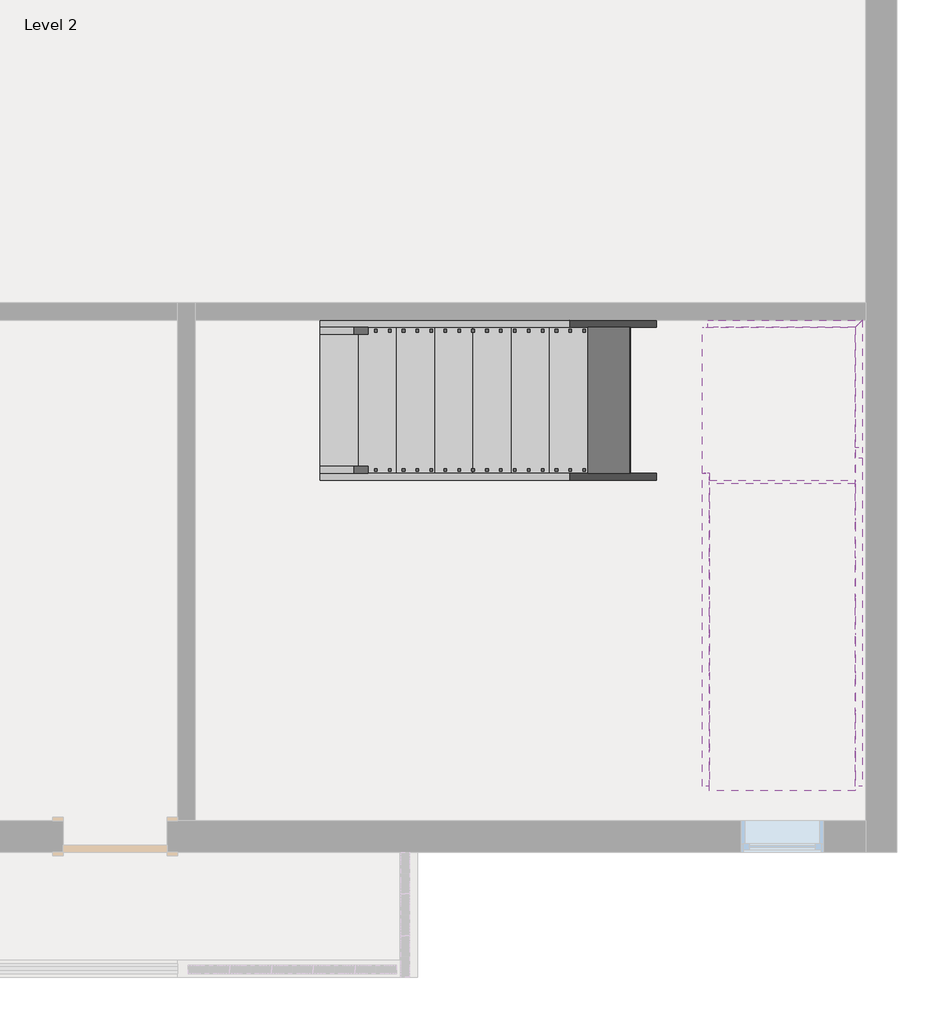
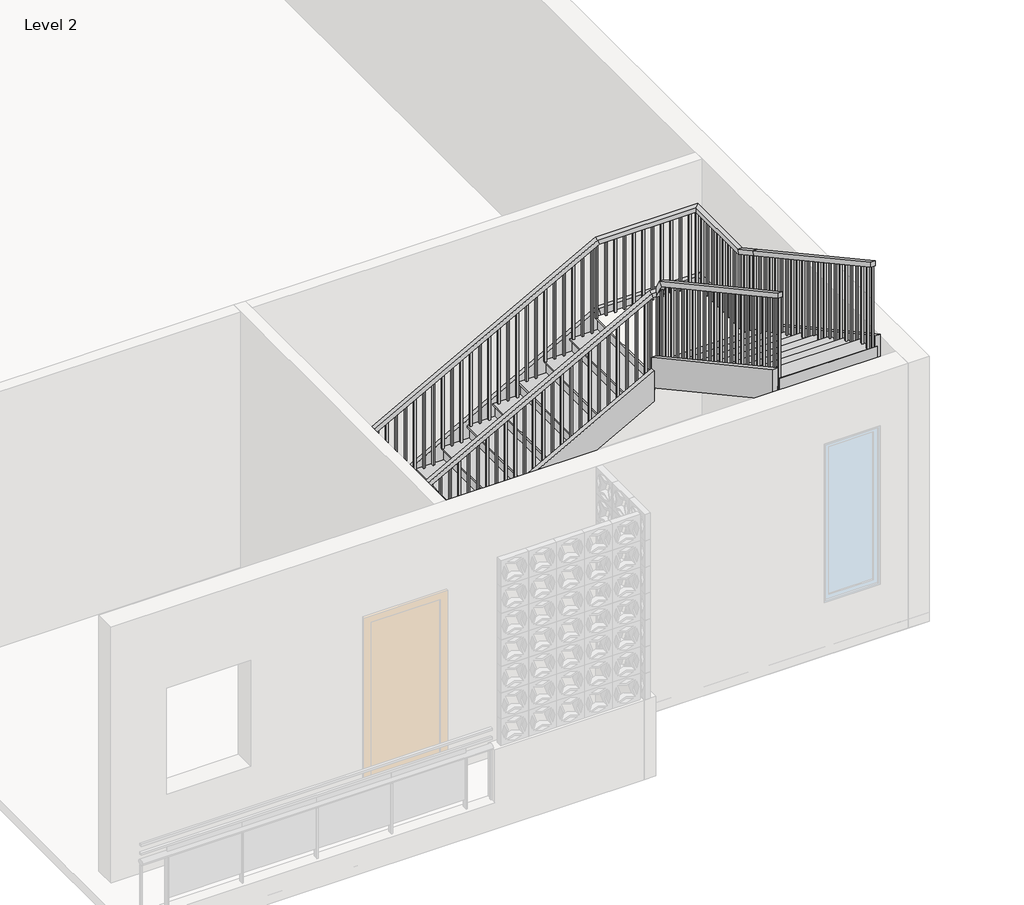
# One storey, part 2 of 2: 6 members, 2 railings, 2 stair flights, 1 slab.
"""IFC4 building model written with IfcOpenShell, lengths in millimetres."""

from ifc_helpers import new_model, si_unit, frame, origin, place, context, project, spatial, polyline, outline, extrude, faceted_brep, transform, mapped, element, save
from components import non_monolithic_landing_9b4a1add, stair_flight_2c29bb35, stair_flight_8fbc4922

model = new_model("IFC4")

# Units and contexts
model_context = context("Model", 3, world=origin())
ifc_project = project(units=[si_unit("LENGTHUNIT", "METRE", prefix="MILLI")], contexts=[model_context])

# Site, building, storey
site = spatial("IfcSite", under=ifc_project)
building = spatial("IfcBuilding", under=site)
storey = spatial("IfcBuildingStorey", under=building, Name="Level 2", Elevation=3048.0)

# Members
placement = place(None, origin())
element("IfcMember", 1, ObjectType="Stringer - 2\" Width", at=placement, inside=storey, context=model_context, shape_type="SweptSolid", body=[
    extrude(outline(polyline([(3254.7436667, -459.26646), (3048.0, -459.26646), (3048.0, -201.7743401), (4495.8, 2452.5256599), (4800.6, 2374.8034844), (3254.7436667, -459.26646)])), frame((0.0, -782.3834702, 0.0), z_axis=(0.0, 1.0, 0.0), x_axis=(0.0, 0.0, 1.0)), (0.0, 0.0, 1.0), 50.8),
])
element("IfcMember", 2, ObjectType="Stringer - 2\" Width", at=placement, inside=storey, context=model_context, shape_type="SweptSolid", body=[
    extrude(outline(polyline([(3254.7436667, -459.26646), (3048.0, -459.26646), (3048.0, -201.7743401), (4431.5497528, 2334.73354), (4778.7436667, 2334.73354), (3254.7436667, -459.26646)])), frame((0.0, -1899.9834702, 0.0), z_axis=(0.0, 1.0, 0.0), x_axis=(0.0, 0.0, 1.0)), (0.0, 0.0, 1.0), 50.8),
])
element("IfcMember", 3, ObjectType="Stringer - 2\" Width", at=placement, inside=storey, context=model_context, shape_type="SweptSolid", body=[
    extrude(outline(polyline([(-1660.6534146, 4800.6), (-1738.3755901, 4495.8), (-4135.1834702, 5803.1497528), (-4135.1834702, 6150.3436667), (-1660.6534146, 4800.6)])), frame((3452.33354, 0.0, 0.0), z_axis=(1.0, 0.0, 0.0), x_axis=(0.0, 1.0, 0.0)), (0.0, 0.0, 1.0), 50.8),
])
element("IfcMember", 4, ObjectType="Stringer - 2\" Width", at=placement, inside=storey, context=model_context, shape_type="SweptSolid", body=[
    extrude(outline(polyline([(-1849.1834702, 4903.4345758), (-1849.1834702, 4556.2406619), (-4135.1834702, 5803.1497528), (-4135.1834702, 6150.3436667), (-1849.1834702, 4903.4345758)])), frame((2334.73354, 0.0, 0.0), z_axis=(1.0, 0.0, 0.0), x_axis=(0.0, 1.0, 0.0)), (0.0, 0.0, 1.0), 50.8),
])
element("IfcMember", 5, ObjectType="Stringer - 2\" Width", at=placement, inside=storey, context=model_context, shape_type="Brep", body=[
    faceted_brep([(3452.33354, -1660.6534146, 4800.6), (3503.13354, -1660.6534146, 4800.6), (3503.13354, -731.5834702, 4800.6), (3452.33354, -782.3834702, 4800.6), (3452.33354, -1738.3755901, 4495.8), (3452.33354, -782.3834702, 4495.8), (3503.13354, -1738.3755901, 4495.8), (3503.13354, -731.5834702, 4495.8)], [[[0, 1, 2, 3]], [[4, 0, 3, 5]], [[6, 4, 5, 7]], [[1, 6, 7, 2]], [[1, 0, 4, 6]], [[2, 7, 5, 3]]]),
])
element("IfcMember", 6, ObjectType="Stringer - 2\" Width", at=placement, inside=storey, context=model_context, shape_type="Brep", body=[
    faceted_brep([(3452.33354, -782.3834702, 4800.6), (3503.13354, -731.5834702, 4800.6), (2374.8034844, -731.5834702, 4800.6), (2374.8034844, -782.3834702, 4800.6), (3452.33354, -782.3834702, 4495.8), (2452.5256599, -782.3834702, 4495.8), (3503.13354, -731.5834702, 4495.8), (2452.5256599, -731.5834702, 4495.8)], [[[0, 1, 2, 3]], [[4, 0, 3, 5]], [[6, 4, 5, 7]], [[1, 6, 7, 2]], [[1, 0, 4, 6]], [[2, 7, 5, 3]]]),
])

# Railings
element("IfcRailing", 7, ObjectType="Handrail - Rectangular", at=placement, inside=storey, context=model_context, shape_type="SolidModel", body=[
    faceted_brep([(-459.26646, -1798.3834702, 4114.8), (-459.26646, -1798.3834702, 4056.9343477), (-459.26646, -1849.1834702, 4056.9343477), (-459.26646, -1849.1834702, 4114.8), (2334.73354, -1798.3834702, 5638.8), (2347.687236, -1798.3834702, 5588.0), (2347.687236, -1849.1834702, 5588.0), (2334.73354, -1849.1834702, 5638.8), (2436.33354, -1798.3834702, 5638.8), (2436.33354, -1849.1834702, 5638.8), (2436.33354, -1849.1834702, 5588.0), (2436.33354, -1798.3834702, 5588.0)], [[[0, 1, 2, 3]], [[1, 0, 4, 5]], [[2, 1, 5, 6]], [[3, 2, 6, 7]], [[0, 3, 7, 4]], [[8, 9, 10, 11]], [[5, 4, 8, 11]], [[6, 5, 11, 10]], [[7, 6, 10, 9]], [[4, 7, 9, 8]]]),
    faceted_brep([(2436.33354, -1849.1834702, 5689.6), (2436.33354, -1849.1834702, 5576.0077467), (2385.53354, -1849.1834702, 5576.0077467), (2385.53354, -1849.1834702, 5689.6), (2436.33354, -1899.9834702, 5791.2), (2436.33354, -1938.2955084, 5754.231823), (2385.53354, -1938.2955084, 5754.231823), (2385.53354, -1899.9834702, 5791.2), (2436.33354, -4135.1834702, 7010.4), (2385.53354, -4135.1834702, 7010.4), (2385.53354, -4135.1834702, 6952.5343477), (2436.33354, -4135.1834702, 6952.5343477)], [[[0, 1, 2, 3]], [[1, 0, 4, 5]], [[2, 1, 5, 6]], [[3, 2, 6, 7]], [[0, 3, 7, 4]], [[8, 9, 10, 11]], [[5, 4, 8, 11]], [[6, 5, 11, 10]], [[7, 6, 10, 9]], [[4, 7, 9, 8]]]),
    extrude(outline(polyline([(-4043.1084702, 6902.3116204), (-4024.0584702, 6891.9207113), (-4024.0584702, 5943.6), (-4043.1084702, 5943.6), (-4043.1084702, 6902.3116204)])), frame((2401.40854, 0.0, 0.0), z_axis=(1.0, 0.0, 0.0), x_axis=(0.0, 1.0, 0.0)), (0.0, 0.0, 1.0), 19.05),
    extrude(outline(polyline([(-3941.5084702, 6846.8934386), (-3922.4584702, 6836.5025295), (-3922.4584702, 5943.6), (-3941.5084702, 5943.6), (-3941.5084702, 6846.8934386)])), frame((2401.40854, 0.0, 0.0), z_axis=(1.0, 0.0, 0.0), x_axis=(0.0, 1.0, 0.0)), (0.0, 0.0, 1.0), 19.05),
    extrude(outline(polyline([(-3839.9084702, 6791.4752568), (-3820.8584702, 6781.0843477), (-3820.8584702, 5791.2), (-3839.9084702, 5791.2), (-3839.9084702, 6791.4752568)])), frame((2401.40854, 0.0, 0.0), z_axis=(1.0, 0.0, 0.0), x_axis=(0.0, 1.0, 0.0)), (0.0, 0.0, 1.0), 19.05),
    extrude(outline(polyline([(-3738.3084702, 6736.0570749), (-3719.2584702, 6725.6661659), (-3719.2584702, 5791.2), (-3738.3084702, 5791.2), (-3738.3084702, 6736.0570749)])), frame((2401.40854, 0.0, 0.0), z_axis=(1.0, 0.0, 0.0), x_axis=(0.0, 1.0, 0.0)), (0.0, 0.0, 1.0), 19.05),
    extrude(outline(polyline([(-3636.7084702, 6680.6388931), (-3617.6584702, 6670.247984), (-3617.6584702, 5791.2), (-3636.7084702, 5791.2), (-3636.7084702, 6680.6388931)])), frame((2401.40854, 0.0, 0.0), z_axis=(1.0, 0.0, 0.0), x_axis=(0.0, 1.0, 0.0)), (0.0, 0.0, 1.0), 19.05),
    extrude(outline(polyline([(-3535.1084702, 6625.2207113), (-3516.0584702, 6614.8298022), (-3516.0584702, 5638.8), (-3535.1084702, 5638.8), (-3535.1084702, 6625.2207113)])), frame((2401.40854, 0.0, 0.0), z_axis=(1.0, 0.0, 0.0), x_axis=(0.0, 1.0, 0.0)), (0.0, 0.0, 1.0), 19.05),
    extrude(outline(polyline([(-3433.5084702, 6569.8025295), (-3414.4584702, 6559.4116204), (-3414.4584702, 5638.8), (-3433.5084702, 5638.8), (-3433.5084702, 6569.8025295)])), frame((2401.40854, 0.0, 0.0), z_axis=(1.0, 0.0, 0.0), x_axis=(0.0, 1.0, 0.0)), (0.0, 0.0, 1.0), 19.05),
    extrude(outline(polyline([(-3331.9084702, 6514.3843477), (-3312.8584702, 6503.9934386), (-3312.8584702, 5638.8), (-3331.9084702, 5638.8), (-3331.9084702, 6514.3843477)])), frame((2401.40854, 0.0, 0.0), z_axis=(1.0, 0.0, 0.0), x_axis=(0.0, 1.0, 0.0)), (0.0, 0.0, 1.0), 19.05),
    extrude(outline(polyline([(-3230.3084702, 6458.9661659), (-3211.2584702, 6448.5752568), (-3211.2584702, 5486.4), (-3230.3084702, 5486.4), (-3230.3084702, 6458.9661659)])), frame((2401.40854, 0.0, 0.0), z_axis=(1.0, 0.0, 0.0), x_axis=(0.0, 1.0, 0.0)), (0.0, 0.0, 1.0), 19.05),
    extrude(outline(polyline([(-3128.7084702, 6403.547984), (-3109.6584702, 6393.1570749), (-3109.6584702, 5486.4), (-3128.7084702, 5486.4), (-3128.7084702, 6403.547984)])), frame((2401.40854, 0.0, 0.0), z_axis=(1.0, 0.0, 0.0), x_axis=(0.0, 1.0, 0.0)), (0.0, 0.0, 1.0), 19.05),
    extrude(outline(polyline([(-3027.1084702, 6348.1298022), (-3008.0584702, 6337.7388931), (-3008.0584702, 5486.4), (-3027.1084702, 5486.4), (-3027.1084702, 6348.1298022)])), frame((2401.40854, 0.0, 0.0), z_axis=(1.0, 0.0, 0.0), x_axis=(0.0, 1.0, 0.0)), (0.0, 0.0, 1.0), 19.05),
    extrude(outline(polyline([(-2925.5084702, 6292.7116204), (-2906.4584702, 6282.3207113), (-2906.4584702, 5334.0), (-2925.5084702, 5334.0), (-2925.5084702, 6292.7116204)])), frame((2401.40854, 0.0, 0.0), z_axis=(1.0, 0.0, 0.0), x_axis=(0.0, 1.0, 0.0)), (0.0, 0.0, 1.0), 19.05),
    extrude(outline(polyline([(-2823.9084702, 6237.2934386), (-2804.8584702, 6226.9025295), (-2804.8584702, 5334.0), (-2823.9084702, 5334.0), (-2823.9084702, 6237.2934386)])), frame((2401.40854, 0.0, 0.0), z_axis=(1.0, 0.0, 0.0), x_axis=(0.0, 1.0, 0.0)), (0.0, 0.0, 1.0), 19.05),
    extrude(outline(polyline([(-2722.3084702, 6181.8752568), (-2703.2584702, 6171.4843477), (-2703.2584702, 5181.6), (-2722.3084702, 5181.6), (-2722.3084702, 6181.8752568)])), frame((2401.40854, 0.0, 0.0), z_axis=(1.0, 0.0, 0.0), x_axis=(0.0, 1.0, 0.0)), (0.0, 0.0, 1.0), 19.05),
    extrude(outline(polyline([(-2620.7084702, 6126.4570749), (-2601.6584702, 6116.0661659), (-2601.6584702, 5181.6), (-2620.7084702, 5181.6), (-2620.7084702, 6126.4570749)])), frame((2401.40854, 0.0, 0.0), z_axis=(1.0, 0.0, 0.0), x_axis=(0.0, 1.0, 0.0)), (0.0, 0.0, 1.0), 19.05),
    extrude(outline(polyline([(-2519.1084702, 6071.0388931), (-2500.0584702, 6060.647984), (-2500.0584702, 5181.6), (-2519.1084702, 5181.6), (-2519.1084702, 6071.0388931)])), frame((2401.40854, 0.0, 0.0), z_axis=(1.0, 0.0, 0.0), x_axis=(0.0, 1.0, 0.0)), (0.0, 0.0, 1.0), 19.05),
    extrude(outline(polyline([(-2417.5084702, 6015.6207113), (-2398.4584702, 6005.2298022), (-2398.4584702, 5029.2), (-2417.5084702, 5029.2), (-2417.5084702, 6015.6207113)])), frame((2401.40854, 0.0, 0.0), z_axis=(1.0, 0.0, 0.0), x_axis=(0.0, 1.0, 0.0)), (0.0, 0.0, 1.0), 19.05),
    extrude(outline(polyline([(-2315.9084702, 5960.2025295), (-2296.8584702, 5949.8116204), (-2296.8584702, 5029.2), (-2315.9084702, 5029.2), (-2315.9084702, 5960.2025295)])), frame((2401.40854, 0.0, 0.0), z_axis=(1.0, 0.0, 0.0), x_axis=(0.0, 1.0, 0.0)), (0.0, 0.0, 1.0), 19.05),
    extrude(outline(polyline([(-2214.3084702, 5904.7843477), (-2195.2584702, 5894.3934386), (-2195.2584702, 5029.2), (-2214.3084702, 5029.2), (-2214.3084702, 5904.7843477)])), frame((2401.40854, 0.0, 0.0), z_axis=(1.0, 0.0, 0.0), x_axis=(0.0, 1.0, 0.0)), (0.0, 0.0, 1.0), 19.05),
    extrude(outline(polyline([(-2112.7084702, 5849.3661659), (-2093.6584702, 5838.9752568), (-2093.6584702, 4876.8), (-2112.7084702, 4876.8), (-2112.7084702, 5849.3661659)])), frame((2401.40854, 0.0, 0.0), z_axis=(1.0, 0.0, 0.0), x_axis=(0.0, 1.0, 0.0)), (0.0, 0.0, 1.0), 19.05),
    extrude(outline(polyline([(-2011.1084702, 5793.947984), (-1992.0584702, 5783.5570749), (-1992.0584702, 4876.8), (-2011.1084702, 4876.8), (-2011.1084702, 5793.947984)])), frame((2401.40854, 0.0, 0.0), z_axis=(1.0, 0.0, 0.0), x_axis=(0.0, 1.0, 0.0)), (0.0, 0.0, 1.0), 19.05),
    extrude(outline(polyline([(5558.4207113, 2293.45854), (5548.0298022, 2274.40854), (4572.0, 2274.40854), (4572.0, 2293.45854), (5558.4207113, 2293.45854)])), frame((0.0, -1833.3084702, 0.0), z_axis=(0.0, 1.0, 0.0), x_axis=(0.0, 0.0, 1.0)), (0.0, 0.0, 1.0), 19.05),
    extrude(outline(polyline([(5503.0025295, 2191.85854), (5492.6116204, 2172.80854), (4572.0, 2172.80854), (4572.0, 2191.85854), (5503.0025295, 2191.85854)])), frame((0.0, -1833.3084702, 0.0), z_axis=(0.0, 1.0, 0.0), x_axis=(0.0, 0.0, 1.0)), (0.0, 0.0, 1.0), 19.05),
    extrude(outline(polyline([(5447.5843477, 2090.25854), (5437.1934386, 2071.20854), (4572.0, 2071.20854), (4572.0, 2090.25854), (5447.5843477, 2090.25854)])), frame((0.0, -1833.3084702, 0.0), z_axis=(0.0, 1.0, 0.0), x_axis=(0.0, 0.0, 1.0)), (0.0, 0.0, 1.0), 19.05),
    extrude(outline(polyline([(5392.1661659, 1988.65854), (5381.7752568, 1969.60854), (4419.6, 1969.60854), (4419.6, 1988.65854), (5392.1661659, 1988.65854)])), frame((0.0, -1833.3084702, 0.0), z_axis=(0.0, 1.0, 0.0), x_axis=(0.0, 0.0, 1.0)), (0.0, 0.0, 1.0), 19.05),
    extrude(outline(polyline([(5336.747984, 1887.05854), (5326.3570749, 1868.00854), (4419.6, 1868.00854), (4419.6, 1887.05854), (5336.747984, 1887.05854)])), frame((0.0, -1833.3084702, 0.0), z_axis=(0.0, 1.0, 0.0), x_axis=(0.0, 0.0, 1.0)), (0.0, 0.0, 1.0), 19.05),
    extrude(outline(polyline([(5281.3298022, 1785.45854), (5270.9388931, 1766.40854), (4419.6, 1766.40854), (4419.6, 1785.45854), (5281.3298022, 1785.45854)])), frame((0.0, -1833.3084702, 0.0), z_axis=(0.0, 1.0, 0.0), x_axis=(0.0, 0.0, 1.0)), (0.0, 0.0, 1.0), 19.05),
    extrude(outline(polyline([(5225.9116204, 1683.85854), (5215.5207113, 1664.80854), (4267.2, 1664.80854), (4267.2, 1683.85854), (5225.9116204, 1683.85854)])), frame((0.0, -1833.3084702, 0.0), z_axis=(0.0, 1.0, 0.0), x_axis=(0.0, 0.0, 1.0)), (0.0, 0.0, 1.0), 19.05),
    extrude(outline(polyline([(5170.4934386, 1582.25854), (5160.1025295, 1563.20854), (4267.2, 1563.20854), (4267.2, 1582.25854), (5170.4934386, 1582.25854)])), frame((0.0, -1833.3084702, 0.0), z_axis=(0.0, 1.0, 0.0), x_axis=(0.0, 0.0, 1.0)), (0.0, 0.0, 1.0), 19.05),
    extrude(outline(polyline([(5115.0752568, 1480.65854), (5104.6843477, 1461.60854), (4114.8, 1461.60854), (4114.8, 1480.65854), (5115.0752568, 1480.65854)])), frame((0.0, -1833.3084702, 0.0), z_axis=(0.0, 1.0, 0.0), x_axis=(0.0, 0.0, 1.0)), (0.0, 0.0, 1.0), 19.05),
    extrude(outline(polyline([(5059.6570749, 1379.05854), (5049.2661659, 1360.00854), (4114.8, 1360.00854), (4114.8, 1379.05854), (5059.6570749, 1379.05854)])), frame((0.0, -1833.3084702, 0.0), z_axis=(0.0, 1.0, 0.0), x_axis=(0.0, 0.0, 1.0)), (0.0, 0.0, 1.0), 19.05),
    extrude(outline(polyline([(5004.2388931, 1277.45854), (4993.847984, 1258.40854), (4114.8, 1258.40854), (4114.8, 1277.45854), (5004.2388931, 1277.45854)])), frame((0.0, -1833.3084702, 0.0), z_axis=(0.0, 1.0, 0.0), x_axis=(0.0, 0.0, 1.0)), (0.0, 0.0, 1.0), 19.05),
    extrude(outline(polyline([(4948.8207113, 1175.85854), (4938.4298022, 1156.80854), (3962.4, 1156.80854), (3962.4, 1175.85854), (4948.8207113, 1175.85854)])), frame((0.0, -1833.3084702, 0.0), z_axis=(0.0, 1.0, 0.0), x_axis=(0.0, 0.0, 1.0)), (0.0, 0.0, 1.0), 19.05),
    extrude(outline(polyline([(4893.4025295, 1074.25854), (4883.0116204, 1055.20854), (3962.4, 1055.20854), (3962.4, 1074.25854), (4893.4025295, 1074.25854)])), frame((0.0, -1833.3084702, 0.0), z_axis=(0.0, 1.0, 0.0), x_axis=(0.0, 0.0, 1.0)), (0.0, 0.0, 1.0), 19.05),
    extrude(outline(polyline([(4837.9843477, 972.65854), (4827.5934386, 953.60854), (3962.4, 953.60854), (3962.4, 972.65854), (4837.9843477, 972.65854)])), frame((0.0, -1833.3084702, 0.0), z_axis=(0.0, 1.0, 0.0), x_axis=(0.0, 0.0, 1.0)), (0.0, 0.0, 1.0), 19.05),
    extrude(outline(polyline([(4782.5661659, 871.05854), (4772.1752568, 852.00854), (3810.0, 852.00854), (3810.0, 871.05854), (4782.5661659, 871.05854)])), frame((0.0, -1833.3084702, 0.0), z_axis=(0.0, 1.0, 0.0), x_axis=(0.0, 0.0, 1.0)), (0.0, 0.0, 1.0), 19.05),
    extrude(outline(polyline([(4727.147984, 769.45854), (4716.7570749, 750.40854), (3810.0, 750.40854), (3810.0, 769.45854), (4727.147984, 769.45854)])), frame((0.0, -1833.3084702, 0.0), z_axis=(0.0, 1.0, 0.0), x_axis=(0.0, 0.0, 1.0)), (0.0, 0.0, 1.0), 19.05),
    extrude(outline(polyline([(4671.7298022, 667.85854), (4661.3388931, 648.80854), (3810.0, 648.80854), (3810.0, 667.85854), (4671.7298022, 667.85854)])), frame((0.0, -1833.3084702, 0.0), z_axis=(0.0, 1.0, 0.0), x_axis=(0.0, 0.0, 1.0)), (0.0, 0.0, 1.0), 19.05),
    extrude(outline(polyline([(4616.3116204, 566.25854), (4605.9207113, 547.20854), (3657.6, 547.20854), (3657.6, 566.25854), (4616.3116204, 566.25854)])), frame((0.0, -1833.3084702, 0.0), z_axis=(0.0, 1.0, 0.0), x_axis=(0.0, 0.0, 1.0)), (0.0, 0.0, 1.0), 19.05),
    extrude(outline(polyline([(4560.8934386, 464.65854), (4550.5025295, 445.60854), (3657.6, 445.60854), (3657.6, 464.65854), (4560.8934386, 464.65854)])), frame((0.0, -1833.3084702, 0.0), z_axis=(0.0, 1.0, 0.0), x_axis=(0.0, 0.0, 1.0)), (0.0, 0.0, 1.0), 19.05),
    extrude(outline(polyline([(4505.4752568, 363.05854), (4495.0843477, 344.00854), (3505.2, 344.00854), (3505.2, 363.05854), (4505.4752568, 363.05854)])), frame((0.0, -1833.3084702, 0.0), z_axis=(0.0, 1.0, 0.0), x_axis=(0.0, 0.0, 1.0)), (0.0, 0.0, 1.0), 19.05),
    extrude(outline(polyline([(4450.0570749, 261.45854), (4439.6661659, 242.40854), (3505.2, 242.40854), (3505.2, 261.45854), (4450.0570749, 261.45854)])), frame((0.0, -1833.3084702, 0.0), z_axis=(0.0, 1.0, 0.0), x_axis=(0.0, 0.0, 1.0)), (0.0, 0.0, 1.0), 19.05),
    extrude(outline(polyline([(4394.6388931, 159.85854), (4384.247984, 140.80854), (3505.2, 140.80854), (3505.2, 159.85854), (4394.6388931, 159.85854)])), frame((0.0, -1833.3084702, 0.0), z_axis=(0.0, 1.0, 0.0), x_axis=(0.0, 0.0, 1.0)), (0.0, 0.0, 1.0), 19.05),
    extrude(outline(polyline([(4339.2207113, 58.25854), (4328.8298022, 39.20854), (3352.8, 39.20854), (3352.8, 58.25854), (4339.2207113, 58.25854)])), frame((0.0, -1833.3084702, 0.0), z_axis=(0.0, 1.0, 0.0), x_axis=(0.0, 0.0, 1.0)), (0.0, 0.0, 1.0), 19.05),
    extrude(outline(polyline([(4283.8025295, -43.34146), (4273.4116204, -62.39146), (3352.8, -62.39146), (3352.8, -43.34146), (4283.8025295, -43.34146)])), frame((0.0, -1833.3084702, 0.0), z_axis=(0.0, 1.0, 0.0), x_axis=(0.0, 0.0, 1.0)), (0.0, 0.0, 1.0), 19.05),
    extrude(outline(polyline([(4228.3843477, -144.94146), (4217.9934386, -163.99146), (3352.8, -163.99146), (3352.8, -144.94146), (4228.3843477, -144.94146)])), frame((0.0, -1833.3084702, 0.0), z_axis=(0.0, 1.0, 0.0), x_axis=(0.0, 0.0, 1.0)), (0.0, 0.0, 1.0), 19.05),
    extrude(outline(polyline([(4172.9661659, -246.54146), (4162.5752568, -265.59146), (3200.4, -265.59146), (3200.4, -246.54146), (4172.9661659, -246.54146)])), frame((0.0, -1833.3084702, 0.0), z_axis=(0.0, 1.0, 0.0), x_axis=(0.0, 0.0, 1.0)), (0.0, 0.0, 1.0), 19.05),
    extrude(outline(polyline([(4117.547984, -348.14146), (4107.1570749, -367.19146), (3200.4, -367.19146), (3200.4, -348.14146), (4117.547984, -348.14146)])), frame((0.0, -1833.3084702, 0.0), z_axis=(0.0, 1.0, 0.0), x_axis=(0.0, 0.0, 1.0)), (0.0, 0.0, 1.0), 19.05),
    extrude(outline(polyline([(-1909.5084702, 5696.6577467), (-1890.4584702, 5658.5577467), (-1890.4584702, 4724.4), (-1909.5084702, 4724.4), (-1909.5084702, 5696.6577467)])), frame((2401.40854, 0.0, 0.0), z_axis=(1.0, 0.0, 0.0), x_axis=(0.0, 1.0, 0.0)), (0.0, 0.0, 1.0), 19.05),
    extrude(outline(polyline([(2401.40854, -1833.3084702), (2401.40854, -1814.2584702), (2420.45854, -1814.2584702), (2420.45854, -1833.3084702), (2401.40854, -1833.3084702)])), frame((0.0, 0.0, 4724.4), z_axis=(0.0, 0.0, 1.0), x_axis=(1.0, 0.0, 0.0)), (0.0, 0.0, 1.0), 863.6),
    extrude(outline(polyline([(5586.1298022, 2344.25854), (5575.7388931, 2325.20854), (4724.4, 2325.20854), (4724.4, 2344.25854), (5586.1298022, 2344.25854)])), frame((0.0, -1833.3084702, 0.0), z_axis=(0.0, 1.0, 0.0), x_axis=(0.0, 0.0, 1.0)), (0.0, 0.0, 1.0), 19.05),
    extrude(outline(polyline([(-4135.1834702, 6952.5343477), (-4116.1334702, 6942.1434386), (-4116.1334702, 5943.6), (-4135.1834702, 5943.6), (-4135.1834702, 6952.5343477)])), frame((2401.40854, 0.0, 0.0), z_axis=(1.0, 0.0, 0.0), x_axis=(0.0, 1.0, 0.0)), (0.0, 0.0, 1.0), 19.05),
    extrude(outline(polyline([(4067.3252568, -440.21646), (4056.9343477, -459.26646), (3200.4, -459.26646), (3200.4, -440.21646), (4067.3252568, -440.21646)])), frame((0.0, -1833.3084702, 0.0), z_axis=(0.0, 1.0, 0.0), x_axis=(0.0, 0.0, 1.0)), (0.0, 0.0, 1.0), 19.05),
])
element("IfcRailing", 8, ObjectType="Handrail - Rectangular", at=placement, inside=storey, context=model_context, shape_type="SolidModel", body=[
    faceted_brep([(-459.26646, -782.3834702, 4114.8), (-459.26646, -782.3834702, 4056.9343477), (-459.26646, -833.1834702, 4056.9343477), (-459.26646, -833.1834702, 4114.8), (2334.73354, -782.3834702, 5638.8), (2347.687236, -782.3834702, 5588.0), (2347.687236, -833.1834702, 5588.0), (2334.73354, -833.1834702, 5638.8), (3452.33354, -782.3834702, 5638.8), (3452.33354, -782.3834702, 5588.0), (3401.53354, -833.1834702, 5588.0), (3401.53354, -833.1834702, 5638.8), (3452.33354, -1620.5834702, 5638.8), (3452.33354, -1633.5371661, 5588.0), (3401.53354, -1633.5371661, 5588.0), (3401.53354, -1620.5834702, 5638.8), (3452.33354, -1899.9834702, 5791.2), (3452.33354, -1924.3091585, 5746.6029049), (3401.53354, -1924.3091585, 5746.6029049), (3401.53354, -1899.9834702, 5791.2), (3452.33354, -4135.1834702, 7010.4), (3401.53354, -4135.1834702, 7010.4), (3401.53354, -4135.1834702, 6952.5343477), (3452.33354, -4135.1834702, 6952.5343477)], [[[0, 1, 2, 3]], [[1, 0, 4, 5]], [[2, 1, 5, 6]], [[3, 2, 6, 7]], [[0, 3, 7, 4]], [[5, 4, 8, 9]], [[6, 5, 9, 10]], [[7, 6, 10, 11]], [[4, 7, 11, 8]], [[9, 8, 12, 13]], [[10, 9, 13, 14]], [[11, 10, 14, 15]], [[8, 11, 15, 12]], [[13, 12, 16, 17]], [[14, 13, 17, 18]], [[15, 14, 18, 19]], [[12, 15, 19, 16]], [[20, 21, 22, 23]], [[17, 16, 20, 23]], [[18, 17, 23, 22]], [[19, 18, 22, 21]], [[16, 19, 21, 20]]]),
    extrude(outline(polyline([(-4024.0584702, 6891.9207113), (-4024.0584702, 5943.6), (-4043.1084702, 5943.6), (-4043.1084702, 6902.3116204), (-4024.0584702, 6891.9207113)])), frame((3417.40854, 0.0, 0.0), z_axis=(1.0, 0.0, 0.0), x_axis=(0.0, 1.0, 0.0)), (0.0, 0.0, 1.0), 19.05),
    extrude(outline(polyline([(-3922.4584702, 6836.5025295), (-3922.4584702, 5943.6), (-3941.5084702, 5943.6), (-3941.5084702, 6846.8934386), (-3922.4584702, 6836.5025295)])), frame((3417.40854, 0.0, 0.0), z_axis=(1.0, 0.0, 0.0), x_axis=(0.0, 1.0, 0.0)), (0.0, 0.0, 1.0), 19.05),
    extrude(outline(polyline([(-3820.8584702, 6781.0843477), (-3820.8584702, 5791.2), (-3839.9084702, 5791.2), (-3839.9084702, 6791.4752568), (-3820.8584702, 6781.0843477)])), frame((3417.40854, 0.0, 0.0), z_axis=(1.0, 0.0, 0.0), x_axis=(0.0, 1.0, 0.0)), (0.0, 0.0, 1.0), 19.05),
    extrude(outline(polyline([(-3719.2584702, 6725.6661659), (-3719.2584702, 5791.2), (-3738.3084702, 5791.2), (-3738.3084702, 6736.0570749), (-3719.2584702, 6725.6661659)])), frame((3417.40854, 0.0, 0.0), z_axis=(1.0, 0.0, 0.0), x_axis=(0.0, 1.0, 0.0)), (0.0, 0.0, 1.0), 19.05),
    extrude(outline(polyline([(-3617.6584702, 6670.247984), (-3617.6584702, 5791.2), (-3636.7084702, 5791.2), (-3636.7084702, 6680.6388931), (-3617.6584702, 6670.247984)])), frame((3417.40854, 0.0, 0.0), z_axis=(1.0, 0.0, 0.0), x_axis=(0.0, 1.0, 0.0)), (0.0, 0.0, 1.0), 19.05),
    extrude(outline(polyline([(-3516.0584702, 6614.8298022), (-3516.0584702, 5638.8), (-3535.1084702, 5638.8), (-3535.1084702, 6625.2207113), (-3516.0584702, 6614.8298022)])), frame((3417.40854, 0.0, 0.0), z_axis=(1.0, 0.0, 0.0), x_axis=(0.0, 1.0, 0.0)), (0.0, 0.0, 1.0), 19.05),
    extrude(outline(polyline([(-3414.4584702, 6559.4116204), (-3414.4584702, 5638.8), (-3433.5084702, 5638.8), (-3433.5084702, 6569.8025295), (-3414.4584702, 6559.4116204)])), frame((3417.40854, 0.0, 0.0), z_axis=(1.0, 0.0, 0.0), x_axis=(0.0, 1.0, 0.0)), (0.0, 0.0, 1.0), 19.05),
    extrude(outline(polyline([(-3312.8584702, 6503.9934386), (-3312.8584702, 5638.8), (-3331.9084702, 5638.8), (-3331.9084702, 6514.3843477), (-3312.8584702, 6503.9934386)])), frame((3417.40854, 0.0, 0.0), z_axis=(1.0, 0.0, 0.0), x_axis=(0.0, 1.0, 0.0)), (0.0, 0.0, 1.0), 19.05),
    extrude(outline(polyline([(-3211.2584702, 6448.5752568), (-3211.2584702, 5486.4), (-3230.3084702, 5486.4), (-3230.3084702, 6458.9661659), (-3211.2584702, 6448.5752568)])), frame((3417.40854, 0.0, 0.0), z_axis=(1.0, 0.0, 0.0), x_axis=(0.0, 1.0, 0.0)), (0.0, 0.0, 1.0), 19.05),
    extrude(outline(polyline([(-3109.6584702, 6393.1570749), (-3109.6584702, 5486.4), (-3128.7084702, 5486.4), (-3128.7084702, 6403.547984), (-3109.6584702, 6393.1570749)])), frame((3417.40854, 0.0, 0.0), z_axis=(1.0, 0.0, 0.0), x_axis=(0.0, 1.0, 0.0)), (0.0, 0.0, 1.0), 19.05),
    extrude(outline(polyline([(-3008.0584702, 6337.7388931), (-3008.0584702, 5486.4), (-3027.1084702, 5486.4), (-3027.1084702, 6348.1298022), (-3008.0584702, 6337.7388931)])), frame((3417.40854, 0.0, 0.0), z_axis=(1.0, 0.0, 0.0), x_axis=(0.0, 1.0, 0.0)), (0.0, 0.0, 1.0), 19.05),
    extrude(outline(polyline([(-2906.4584702, 6282.3207113), (-2906.4584702, 5334.0), (-2925.5084702, 5334.0), (-2925.5084702, 6292.7116204), (-2906.4584702, 6282.3207113)])), frame((3417.40854, 0.0, 0.0), z_axis=(1.0, 0.0, 0.0), x_axis=(0.0, 1.0, 0.0)), (0.0, 0.0, 1.0), 19.05),
    extrude(outline(polyline([(-2804.8584702, 6226.9025295), (-2804.8584702, 5334.0), (-2823.9084702, 5334.0), (-2823.9084702, 6237.2934386), (-2804.8584702, 6226.9025295)])), frame((3417.40854, 0.0, 0.0), z_axis=(1.0, 0.0, 0.0), x_axis=(0.0, 1.0, 0.0)), (0.0, 0.0, 1.0), 19.05),
    extrude(outline(polyline([(-2703.2584702, 6171.4843477), (-2703.2584702, 5181.6), (-2722.3084702, 5181.6), (-2722.3084702, 6181.8752568), (-2703.2584702, 6171.4843477)])), frame((3417.40854, 0.0, 0.0), z_axis=(1.0, 0.0, 0.0), x_axis=(0.0, 1.0, 0.0)), (0.0, 0.0, 1.0), 19.05),
    extrude(outline(polyline([(-2601.6584702, 6116.0661659), (-2601.6584702, 5181.6), (-2620.7084702, 5181.6), (-2620.7084702, 6126.4570749), (-2601.6584702, 6116.0661659)])), frame((3417.40854, 0.0, 0.0), z_axis=(1.0, 0.0, 0.0), x_axis=(0.0, 1.0, 0.0)), (0.0, 0.0, 1.0), 19.05),
    extrude(outline(polyline([(-2500.0584702, 6060.647984), (-2500.0584702, 5181.6), (-2519.1084702, 5181.6), (-2519.1084702, 6071.0388931), (-2500.0584702, 6060.647984)])), frame((3417.40854, 0.0, 0.0), z_axis=(1.0, 0.0, 0.0), x_axis=(0.0, 1.0, 0.0)), (0.0, 0.0, 1.0), 19.05),
    extrude(outline(polyline([(-2398.4584702, 6005.2298022), (-2398.4584702, 5029.2), (-2417.5084702, 5029.2), (-2417.5084702, 6015.6207113), (-2398.4584702, 6005.2298022)])), frame((3417.40854, 0.0, 0.0), z_axis=(1.0, 0.0, 0.0), x_axis=(0.0, 1.0, 0.0)), (0.0, 0.0, 1.0), 19.05),
    extrude(outline(polyline([(-2296.8584702, 5949.8116204), (-2296.8584702, 5029.2), (-2315.9084702, 5029.2), (-2315.9084702, 5960.2025295), (-2296.8584702, 5949.8116204)])), frame((3417.40854, 0.0, 0.0), z_axis=(1.0, 0.0, 0.0), x_axis=(0.0, 1.0, 0.0)), (0.0, 0.0, 1.0), 19.05),
    extrude(outline(polyline([(-2195.2584702, 5894.3934386), (-2195.2584702, 5029.2), (-2214.3084702, 5029.2), (-2214.3084702, 5904.7843477), (-2195.2584702, 5894.3934386)])), frame((3417.40854, 0.0, 0.0), z_axis=(1.0, 0.0, 0.0), x_axis=(0.0, 1.0, 0.0)), (0.0, 0.0, 1.0), 19.05),
    extrude(outline(polyline([(-2093.6584702, 5838.9752568), (-2093.6584702, 4876.8), (-2112.7084702, 4876.8), (-2112.7084702, 5849.3661659), (-2093.6584702, 5838.9752568)])), frame((3417.40854, 0.0, 0.0), z_axis=(1.0, 0.0, 0.0), x_axis=(0.0, 1.0, 0.0)), (0.0, 0.0, 1.0), 19.05),
    extrude(outline(polyline([(-1992.0584702, 5783.5570749), (-1992.0584702, 4876.8), (-2011.1084702, 4876.8), (-2011.1084702, 5793.947984), (-1992.0584702, 5783.5570749)])), frame((3417.40854, 0.0, 0.0), z_axis=(1.0, 0.0, 0.0), x_axis=(0.0, 1.0, 0.0)), (0.0, 0.0, 1.0), 19.05),
    extrude(outline(polyline([(-1814.2584702, 5686.5752568), (-1814.2584702, 4724.4), (-1833.3084702, 4724.4), (-1833.3084702, 5696.9661659), (-1814.2584702, 5686.5752568)])), frame((3417.40854, 0.0, 0.0), z_axis=(1.0, 0.0, 0.0), x_axis=(0.0, 1.0, 0.0)), (0.0, 0.0, 1.0), 19.05),
    extrude(outline(polyline([(-1712.6584702, 5631.1570749), (-1712.6584702, 4724.4), (-1731.7084702, 4724.4), (-1731.7084702, 5641.547984), (-1712.6584702, 5631.1570749)])), frame((3417.40854, 0.0, 0.0), z_axis=(1.0, 0.0, 0.0), x_axis=(0.0, 1.0, 0.0)), (0.0, 0.0, 1.0), 19.05),
    extrude(outline(polyline([(3436.45854, -1611.0584702), (3436.45854, -1630.1084702), (3417.40854, -1630.1084702), (3417.40854, -1611.0584702), (3436.45854, -1611.0584702)])), frame((0.0, 0.0, 4724.4), z_axis=(0.0, 0.0, 1.0), x_axis=(1.0, 0.0, 0.0)), (0.0, 0.0, 1.0), 863.6),
    extrude(outline(polyline([(3436.45854, -1509.4584702), (3436.45854, -1528.5084702), (3417.40854, -1528.5084702), (3417.40854, -1509.4584702), (3436.45854, -1509.4584702)])), frame((0.0, 0.0, 4724.4), z_axis=(0.0, 0.0, 1.0), x_axis=(1.0, 0.0, 0.0)), (0.0, 0.0, 1.0), 863.6),
    extrude(outline(polyline([(3436.45854, -1407.8584702), (3436.45854, -1426.9084702), (3417.40854, -1426.9084702), (3417.40854, -1407.8584702), (3436.45854, -1407.8584702)])), frame((0.0, 0.0, 4724.4), z_axis=(0.0, 0.0, 1.0), x_axis=(1.0, 0.0, 0.0)), (0.0, 0.0, 1.0), 863.6),
    extrude(outline(polyline([(3436.45854, -1306.2584702), (3436.45854, -1325.3084702), (3417.40854, -1325.3084702), (3417.40854, -1306.2584702), (3436.45854, -1306.2584702)])), frame((0.0, 0.0, 4724.4), z_axis=(0.0, 0.0, 1.0), x_axis=(1.0, 0.0, 0.0)), (0.0, 0.0, 1.0), 863.6),
    extrude(outline(polyline([(3436.45854, -1204.6584702), (3436.45854, -1223.7084702), (3417.40854, -1223.7084702), (3417.40854, -1204.6584702), (3436.45854, -1204.6584702)])), frame((0.0, 0.0, 4724.4), z_axis=(0.0, 0.0, 1.0), x_axis=(1.0, 0.0, 0.0)), (0.0, 0.0, 1.0), 863.6),
    extrude(outline(polyline([(3436.45854, -1103.0584702), (3436.45854, -1122.1084702), (3417.40854, -1122.1084702), (3417.40854, -1103.0584702), (3436.45854, -1103.0584702)])), frame((0.0, 0.0, 4724.4), z_axis=(0.0, 0.0, 1.0), x_axis=(1.0, 0.0, 0.0)), (0.0, 0.0, 1.0), 863.6),
    extrude(outline(polyline([(3436.45854, -1001.4584702), (3436.45854, -1020.5084702), (3417.40854, -1020.5084702), (3417.40854, -1001.4584702), (3436.45854, -1001.4584702)])), frame((0.0, 0.0, 4724.4), z_axis=(0.0, 0.0, 1.0), x_axis=(1.0, 0.0, 0.0)), (0.0, 0.0, 1.0), 863.6),
    extrude(outline(polyline([(3436.45854, -899.8584702), (3436.45854, -918.9084702), (3417.40854, -918.9084702), (3417.40854, -899.8584702), (3436.45854, -899.8584702)])), frame((0.0, 0.0, 4724.4), z_axis=(0.0, 0.0, 1.0), x_axis=(1.0, 0.0, 0.0)), (0.0, 0.0, 1.0), 863.6),
    extrude(outline(polyline([(3341.20854, -798.2584702), (3360.25854, -798.2584702), (3360.25854, -817.3084702), (3341.20854, -817.3084702), (3341.20854, -798.2584702)])), frame((0.0, 0.0, 4724.4), z_axis=(0.0, 0.0, 1.0), x_axis=(1.0, 0.0, 0.0)), (0.0, 0.0, 1.0), 863.6),
    extrude(outline(polyline([(3239.60854, -798.2584702), (3258.65854, -798.2584702), (3258.65854, -817.3084702), (3239.60854, -817.3084702), (3239.60854, -798.2584702)])), frame((0.0, 0.0, 4724.4), z_axis=(0.0, 0.0, 1.0), x_axis=(1.0, 0.0, 0.0)), (0.0, 0.0, 1.0), 863.6),
    extrude(outline(polyline([(3138.00854, -798.2584702), (3157.05854, -798.2584702), (3157.05854, -817.3084702), (3138.00854, -817.3084702), (3138.00854, -798.2584702)])), frame((0.0, 0.0, 4724.4), z_axis=(0.0, 0.0, 1.0), x_axis=(1.0, 0.0, 0.0)), (0.0, 0.0, 1.0), 863.6),
    extrude(outline(polyline([(3036.40854, -798.2584702), (3055.45854, -798.2584702), (3055.45854, -817.3084702), (3036.40854, -817.3084702), (3036.40854, -798.2584702)])), frame((0.0, 0.0, 4724.4), z_axis=(0.0, 0.0, 1.0), x_axis=(1.0, 0.0, 0.0)), (0.0, 0.0, 1.0), 863.6),
    extrude(outline(polyline([(2934.80854, -798.2584702), (2953.85854, -798.2584702), (2953.85854, -817.3084702), (2934.80854, -817.3084702), (2934.80854, -798.2584702)])), frame((0.0, 0.0, 4724.4), z_axis=(0.0, 0.0, 1.0), x_axis=(1.0, 0.0, 0.0)), (0.0, 0.0, 1.0), 863.6),
    extrude(outline(polyline([(2833.20854, -798.2584702), (2852.25854, -798.2584702), (2852.25854, -817.3084702), (2833.20854, -817.3084702), (2833.20854, -798.2584702)])), frame((0.0, 0.0, 4724.4), z_axis=(0.0, 0.0, 1.0), x_axis=(1.0, 0.0, 0.0)), (0.0, 0.0, 1.0), 863.6),
    extrude(outline(polyline([(2731.60854, -798.2584702), (2750.65854, -798.2584702), (2750.65854, -817.3084702), (2731.60854, -817.3084702), (2731.60854, -798.2584702)])), frame((0.0, 0.0, 4724.4), z_axis=(0.0, 0.0, 1.0), x_axis=(1.0, 0.0, 0.0)), (0.0, 0.0, 1.0), 863.6),
    extrude(outline(polyline([(2630.00854, -798.2584702), (2649.05854, -798.2584702), (2649.05854, -817.3084702), (2630.00854, -817.3084702), (2630.00854, -798.2584702)])), frame((0.0, 0.0, 4724.4), z_axis=(0.0, 0.0, 1.0), x_axis=(1.0, 0.0, 0.0)), (0.0, 0.0, 1.0), 863.6),
    extrude(outline(polyline([(2528.40854, -798.2584702), (2547.45854, -798.2584702), (2547.45854, -817.3084702), (2528.40854, -817.3084702), (2528.40854, -798.2584702)])), frame((0.0, 0.0, 4724.4), z_axis=(0.0, 0.0, 1.0), x_axis=(1.0, 0.0, 0.0)), (0.0, 0.0, 1.0), 863.6),
    extrude(outline(polyline([(2426.80854, -798.2584702), (2445.85854, -798.2584702), (2445.85854, -817.3084702), (2426.80854, -817.3084702), (2426.80854, -798.2584702)])), frame((0.0, 0.0, 4724.4), z_axis=(0.0, 0.0, 1.0), x_axis=(1.0, 0.0, 0.0)), (0.0, 0.0, 1.0), 863.6),
    extrude(outline(polyline([(5548.0298022, 2274.40854), (4572.0, 2274.40854), (4572.0, 2293.45854), (5558.4207113, 2293.45854), (5548.0298022, 2274.40854)])), frame((0.0, -817.3084702, 0.0), z_axis=(0.0, 1.0, 0.0), x_axis=(0.0, 0.0, 1.0)), (0.0, 0.0, 1.0), 19.05),
    extrude(outline(polyline([(5492.6116204, 2172.80854), (4572.0, 2172.80854), (4572.0, 2191.85854), (5503.0025295, 2191.85854), (5492.6116204, 2172.80854)])), frame((0.0, -817.3084702, 0.0), z_axis=(0.0, 1.0, 0.0), x_axis=(0.0, 0.0, 1.0)), (0.0, 0.0, 1.0), 19.05),
    extrude(outline(polyline([(5437.1934386, 2071.20854), (4572.0, 2071.20854), (4572.0, 2090.25854), (5447.5843477, 2090.25854), (5437.1934386, 2071.20854)])), frame((0.0, -817.3084702, 0.0), z_axis=(0.0, 1.0, 0.0), x_axis=(0.0, 0.0, 1.0)), (0.0, 0.0, 1.0), 19.05),
    extrude(outline(polyline([(5381.7752568, 1969.60854), (4419.6, 1969.60854), (4419.6, 1988.65854), (5392.1661659, 1988.65854), (5381.7752568, 1969.60854)])), frame((0.0, -817.3084702, 0.0), z_axis=(0.0, 1.0, 0.0), x_axis=(0.0, 0.0, 1.0)), (0.0, 0.0, 1.0), 19.05),
    extrude(outline(polyline([(5326.3570749, 1868.00854), (4419.6, 1868.00854), (4419.6, 1887.05854), (5336.747984, 1887.05854), (5326.3570749, 1868.00854)])), frame((0.0, -817.3084702, 0.0), z_axis=(0.0, 1.0, 0.0), x_axis=(0.0, 0.0, 1.0)), (0.0, 0.0, 1.0), 19.05),
    extrude(outline(polyline([(5270.9388931, 1766.40854), (4419.6, 1766.40854), (4419.6, 1785.45854), (5281.3298022, 1785.45854), (5270.9388931, 1766.40854)])), frame((0.0, -817.3084702, 0.0), z_axis=(0.0, 1.0, 0.0), x_axis=(0.0, 0.0, 1.0)), (0.0, 0.0, 1.0), 19.05),
    extrude(outline(polyline([(5215.5207113, 1664.80854), (4267.2, 1664.80854), (4267.2, 1683.85854), (5225.9116204, 1683.85854), (5215.5207113, 1664.80854)])), frame((0.0, -817.3084702, 0.0), z_axis=(0.0, 1.0, 0.0), x_axis=(0.0, 0.0, 1.0)), (0.0, 0.0, 1.0), 19.05),
    extrude(outline(polyline([(5160.1025295, 1563.20854), (4267.2, 1563.20854), (4267.2, 1582.25854), (5170.4934386, 1582.25854), (5160.1025295, 1563.20854)])), frame((0.0, -817.3084702, 0.0), z_axis=(0.0, 1.0, 0.0), x_axis=(0.0, 0.0, 1.0)), (0.0, 0.0, 1.0), 19.05),
    extrude(outline(polyline([(5104.6843477, 1461.60854), (4114.8, 1461.60854), (4114.8, 1480.65854), (5115.0752568, 1480.65854), (5104.6843477, 1461.60854)])), frame((0.0, -817.3084702, 0.0), z_axis=(0.0, 1.0, 0.0), x_axis=(0.0, 0.0, 1.0)), (0.0, 0.0, 1.0), 19.05),
    extrude(outline(polyline([(5049.2661659, 1360.00854), (4114.8, 1360.00854), (4114.8, 1379.05854), (5059.6570749, 1379.05854), (5049.2661659, 1360.00854)])), frame((0.0, -817.3084702, 0.0), z_axis=(0.0, 1.0, 0.0), x_axis=(0.0, 0.0, 1.0)), (0.0, 0.0, 1.0), 19.05),
    extrude(outline(polyline([(4993.847984, 1258.40854), (4114.8, 1258.40854), (4114.8, 1277.45854), (5004.2388931, 1277.45854), (4993.847984, 1258.40854)])), frame((0.0, -817.3084702, 0.0), z_axis=(0.0, 1.0, 0.0), x_axis=(0.0, 0.0, 1.0)), (0.0, 0.0, 1.0), 19.05),
    extrude(outline(polyline([(4938.4298022, 1156.80854), (3962.4, 1156.80854), (3962.4, 1175.85854), (4948.8207113, 1175.85854), (4938.4298022, 1156.80854)])), frame((0.0, -817.3084702, 0.0), z_axis=(0.0, 1.0, 0.0), x_axis=(0.0, 0.0, 1.0)), (0.0, 0.0, 1.0), 19.05),
    extrude(outline(polyline([(4883.0116204, 1055.20854), (3962.4, 1055.20854), (3962.4, 1074.25854), (4893.4025295, 1074.25854), (4883.0116204, 1055.20854)])), frame((0.0, -817.3084702, 0.0), z_axis=(0.0, 1.0, 0.0), x_axis=(0.0, 0.0, 1.0)), (0.0, 0.0, 1.0), 19.05),
    extrude(outline(polyline([(4827.5934386, 953.60854), (3962.4, 953.60854), (3962.4, 972.65854), (4837.9843477, 972.65854), (4827.5934386, 953.60854)])), frame((0.0, -817.3084702, 0.0), z_axis=(0.0, 1.0, 0.0), x_axis=(0.0, 0.0, 1.0)), (0.0, 0.0, 1.0), 19.05),
    extrude(outline(polyline([(4772.1752568, 852.00854), (3810.0, 852.00854), (3810.0, 871.05854), (4782.5661659, 871.05854), (4772.1752568, 852.00854)])), frame((0.0, -817.3084702, 0.0), z_axis=(0.0, 1.0, 0.0), x_axis=(0.0, 0.0, 1.0)), (0.0, 0.0, 1.0), 19.05),
    extrude(outline(polyline([(4716.7570749, 750.40854), (3810.0, 750.40854), (3810.0, 769.45854), (4727.147984, 769.45854), (4716.7570749, 750.40854)])), frame((0.0, -817.3084702, 0.0), z_axis=(0.0, 1.0, 0.0), x_axis=(0.0, 0.0, 1.0)), (0.0, 0.0, 1.0), 19.05),
    extrude(outline(polyline([(4661.3388931, 648.80854), (3810.0, 648.80854), (3810.0, 667.85854), (4671.7298022, 667.85854), (4661.3388931, 648.80854)])), frame((0.0, -817.3084702, 0.0), z_axis=(0.0, 1.0, 0.0), x_axis=(0.0, 0.0, 1.0)), (0.0, 0.0, 1.0), 19.05),
    extrude(outline(polyline([(4605.9207113, 547.20854), (3657.6, 547.20854), (3657.6, 566.25854), (4616.3116204, 566.25854), (4605.9207113, 547.20854)])), frame((0.0, -817.3084702, 0.0), z_axis=(0.0, 1.0, 0.0), x_axis=(0.0, 0.0, 1.0)), (0.0, 0.0, 1.0), 19.05),
    extrude(outline(polyline([(4550.5025295, 445.60854), (3657.6, 445.60854), (3657.6, 464.65854), (4560.8934386, 464.65854), (4550.5025295, 445.60854)])), frame((0.0, -817.3084702, 0.0), z_axis=(0.0, 1.0, 0.0), x_axis=(0.0, 0.0, 1.0)), (0.0, 0.0, 1.0), 19.05),
    extrude(outline(polyline([(4495.0843477, 344.00854), (3505.2, 344.00854), (3505.2, 363.05854), (4505.4752568, 363.05854), (4495.0843477, 344.00854)])), frame((0.0, -817.3084702, 0.0), z_axis=(0.0, 1.0, 0.0), x_axis=(0.0, 0.0, 1.0)), (0.0, 0.0, 1.0), 19.05),
    extrude(outline(polyline([(4439.6661659, 242.40854), (3505.2, 242.40854), (3505.2, 261.45854), (4450.0570749, 261.45854), (4439.6661659, 242.40854)])), frame((0.0, -817.3084702, 0.0), z_axis=(0.0, 1.0, 0.0), x_axis=(0.0, 0.0, 1.0)), (0.0, 0.0, 1.0), 19.05),
    extrude(outline(polyline([(4384.247984, 140.80854), (3505.2, 140.80854), (3505.2, 159.85854), (4394.6388931, 159.85854), (4384.247984, 140.80854)])), frame((0.0, -817.3084702, 0.0), z_axis=(0.0, 1.0, 0.0), x_axis=(0.0, 0.0, 1.0)), (0.0, 0.0, 1.0), 19.05),
    extrude(outline(polyline([(4328.8298022, 39.20854), (3352.8, 39.20854), (3352.8, 58.25854), (4339.2207113, 58.25854), (4328.8298022, 39.20854)])), frame((0.0, -817.3084702, 0.0), z_axis=(0.0, 1.0, 0.0), x_axis=(0.0, 0.0, 1.0)), (0.0, 0.0, 1.0), 19.05),
    extrude(outline(polyline([(4273.4116204, -62.39146), (3352.8, -62.39146), (3352.8, -43.34146), (4283.8025295, -43.34146), (4273.4116204, -62.39146)])), frame((0.0, -817.3084702, 0.0), z_axis=(0.0, 1.0, 0.0), x_axis=(0.0, 0.0, 1.0)), (0.0, 0.0, 1.0), 19.05),
    extrude(outline(polyline([(4217.9934386, -163.99146), (3352.8, -163.99146), (3352.8, -144.94146), (4228.3843477, -144.94146), (4217.9934386, -163.99146)])), frame((0.0, -817.3084702, 0.0), z_axis=(0.0, 1.0, 0.0), x_axis=(0.0, 0.0, 1.0)), (0.0, 0.0, 1.0), 19.05),
    extrude(outline(polyline([(4162.5752568, -265.59146), (3200.4, -265.59146), (3200.4, -246.54146), (4172.9661659, -246.54146), (4162.5752568, -265.59146)])), frame((0.0, -817.3084702, 0.0), z_axis=(0.0, 1.0, 0.0), x_axis=(0.0, 0.0, 1.0)), (0.0, 0.0, 1.0), 19.05),
    extrude(outline(polyline([(4107.1570749, -367.19146), (3200.4, -367.19146), (3200.4, -348.14146), (4117.547984, -348.14146), (4107.1570749, -367.19146)])), frame((0.0, -817.3084702, 0.0), z_axis=(0.0, 1.0, 0.0), x_axis=(0.0, 0.0, 1.0)), (0.0, 0.0, 1.0), 19.05),
    extrude(outline(polyline([(-1890.4584702, 5728.1388931), (-1890.4584702, 4724.4), (-1909.5084702, 4724.4), (-1909.5084702, 5738.5298022), (-1890.4584702, 5728.1388931)])), frame((3417.40854, 0.0, 0.0), z_axis=(1.0, 0.0, 0.0), x_axis=(0.0, 1.0, 0.0)), (0.0, 0.0, 1.0), 19.05),
    extrude(outline(polyline([(3417.40854, -798.2584702), (3436.45854, -798.2584702), (3436.45854, -817.3084702), (3417.40854, -817.3084702), (3417.40854, -798.2584702)])), frame((0.0, 0.0, 4724.4), z_axis=(0.0, 0.0, 1.0), x_axis=(1.0, 0.0, 0.0)), (0.0, 0.0, 1.0), 863.6),
    extrude(outline(polyline([(5575.7388931, 2325.20854), (4724.4, 2325.20854), (4724.4, 2344.25854), (5586.1298022, 2344.25854), (5575.7388931, 2325.20854)])), frame((0.0, -817.3084702, 0.0), z_axis=(0.0, 1.0, 0.0), x_axis=(0.0, 0.0, 1.0)), (0.0, 0.0, 1.0), 19.05),
    extrude(outline(polyline([(-4116.1334702, 6942.1434386), (-4116.1334702, 5943.6), (-4135.1834702, 5943.6), (-4135.1834702, 6952.5343477), (-4116.1334702, 6942.1434386)])), frame((3417.40854, 0.0, 0.0), z_axis=(1.0, 0.0, 0.0), x_axis=(0.0, 1.0, 0.0)), (0.0, 0.0, 1.0), 19.05),
    extrude(outline(polyline([(4056.9343477, -459.26646), (3200.4, -459.26646), (3200.4, -440.21646), (4067.3252568, -440.21646), (4056.9343477, -459.26646)])), frame((0.0, -817.3084702, 0.0), z_axis=(0.0, 1.0, 0.0), x_axis=(0.0, 0.0, 1.0)), (0.0, 0.0, 1.0), 19.05),
])

# Slab
non_monolithic_landing_shape = non_monolithic_landing_9b4a1add(model_context)
element("IfcSlab", 9, ObjectType="Non-Monolithic Landing", at=placement, inside=storey, context=model_context, shape_type="MappedRepresentation", body=[
    mapped(non_monolithic_landing_shape, transform((0.0, 0.0, 0.0), x_axis=(1.0, 0.0, 0.0), y_axis=(0.0, 1.0, 0.0), z_axis=(0.0, 0.0, 1.0))),
])

# Stair flights
stair_flight_shape = stair_flight_2c29bb35(model_context)
element("IfcStairFlight", 10, ObjectType="2\" Tread 1\" Nosing 1/4\" Riser", at=placement, inside=storey, context=model_context, shape_type="MappedRepresentation", body=[
    mapped(stair_flight_shape, transform((0.0, 0.0, 0.0), x_axis=(1.0, 0.0, 0.0), y_axis=(0.0, 1.0, 0.0), z_axis=(0.0, 0.0, 1.0))),
])
stair_flight_2_shape = stair_flight_8fbc4922(model_context)
element("IfcStairFlight", 11, ObjectType="2\" Tread 1\" Nosing 1/4\" Riser", at=placement, inside=storey, context=model_context, shape_type="MappedRepresentation", body=[
    mapped(stair_flight_2_shape, transform((0.0, 0.0, 0.0), x_axis=(1.0, 0.0, 0.0), y_axis=(0.0, 1.0, 0.0), z_axis=(0.0, 0.0, 1.0))),
])

save(model, "model.ifc")

# Revit data of these elements
# Type "Handrail - Rectangular"
#   Assembly Code = "C2010400"
#   built-in parameter 1008612 = 0.0416667 (stored number, unit not read)
#   built-in parameter 1008611 = 0.0416667 (stored number, unit not read)
#   built-in parameter 1008609 = 0.333333 (stored number, unit not read)
#   built-in parameter 1008604 = 0.166667 (stored number, unit not read)
#   built-in parameter 1008603 = 0.166667 (stored number, unit not read)
#   Railing Height = 3' - 0"
#   built-in parameter 1008630 = 2
#   built-in parameter 1008610 = 2
#   built-in parameter 1008618 = Baluster - Square : 3/4"
# Elements 1, 2, 3, 4, 5, 6 (IfcMember, "Stringer - 2\" Width")
#   Phase Created = New Construction
# Elements 7, 8 (IfcRailing, "Handrail - Rectangular")
#   Phase Created = New Construction
# Element 9 (IfcSlab, "Non-Monolithic Landing")
#   Phase Created = New Construction
# Elements 10, 11 (IfcStairFlight, "2\" Tread 1\" Nosing 1/4\" Riser")
#   Phase Created = New Construction
